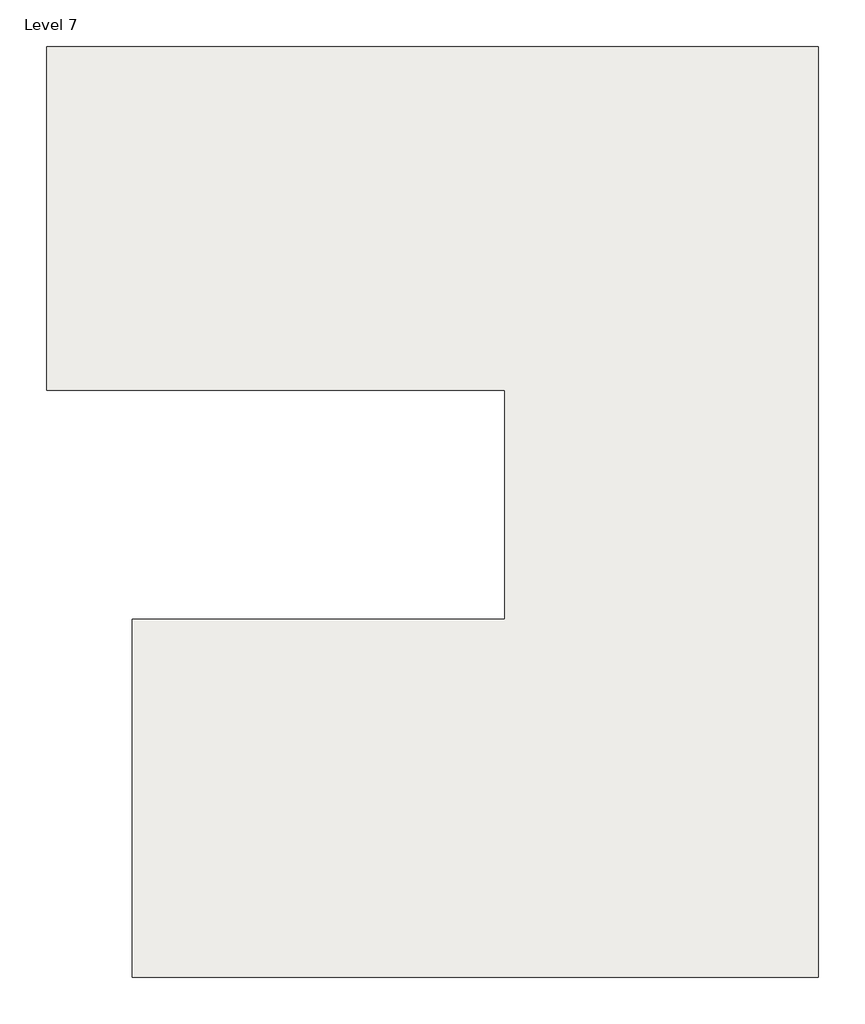
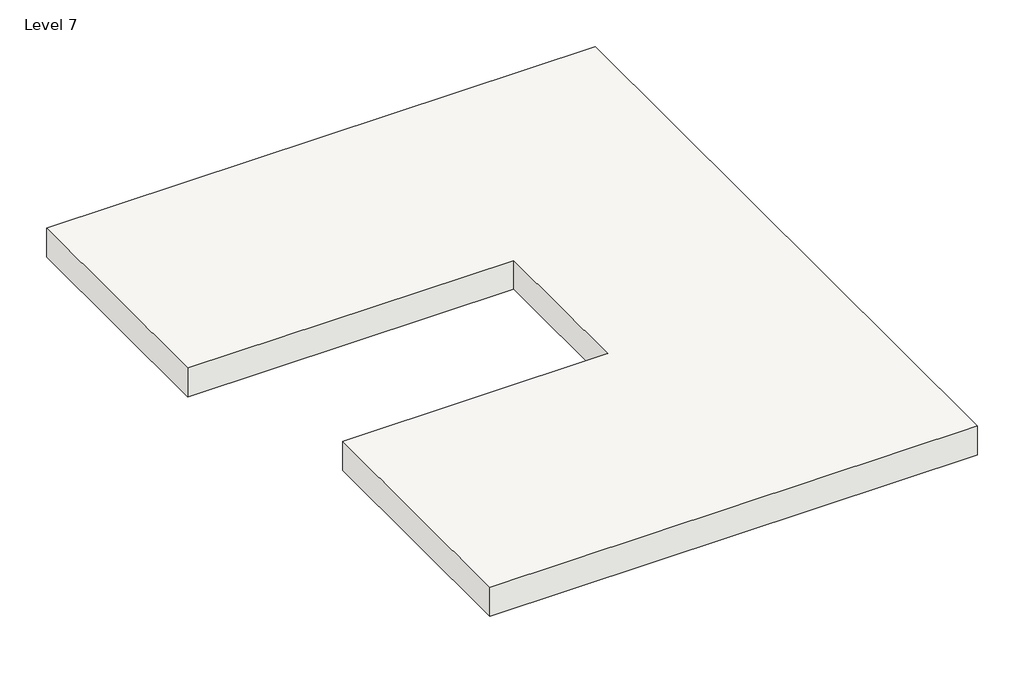
# One storey: 1 slab.
"""IFC4 building model written with IfcOpenShell, lengths in millimetres."""

from ifc_helpers import new_model, si_unit, frame, origin, place, context, project, spatial, polyline, outline, extrude, element, save

model = new_model("IFC4")

# Units and contexts
model_context = context("Model", 3, world=origin())
ifc_project = project(units=[si_unit("LENGTHUNIT", "METRE", prefix="MILLI")], contexts=[model_context])

# Site, building, storey
site = spatial("IfcSite", under=ifc_project)
building = spatial("IfcBuilding", under=site)
storey = spatial("IfcBuildingStorey", under=building, Name="Level 7", Elevation=16154.4)

# Slab
placement = place(None, origin())
element("IfcSlab", 1, ObjectType="Generic - 12\"", at=placement, inside=storey, context=model_context, shape_type="SweptSolid", body=[
    extrude(outline(polyline([(3628.7930349, 1905.6555142), (1196.7430349, 1905.6555142), (1196.7430349, 3175.6555142), (2517.5430349, 3175.6555142), (2517.5430349, 3988.4555142), (891.9430349, 3988.4555142), (891.9430349, 5207.6555142), (3628.7930349, 5207.6555142), (3628.7930349, 1905.6555142)])), frame((0.0, 0.0, 16306.8), z_axis=(0.0, 0.0, 1.0), x_axis=(1.0, 0.0, 0.0)), (0.0, 0.0, 1.0), 152.4),
])

save(model, "model.ifc")

# Revit data of these elements
# Type "Generic - 12\""
#   Assembly Code = "B1010"
#   Function = 0
#   Layers, outside or top first: 0' - 6" no material (function 1)
# Element 1 (IfcSlab, "Generic - 12\"")
#   Height Offset From Level = 1' - 0"
#   Phase Created = New Construction
#   Materials on its faces: "1 wall white"
# Materials
#   "1 wall white": class "Generic", colour RGB 244 245 241, transparency 0, Cost = 0
